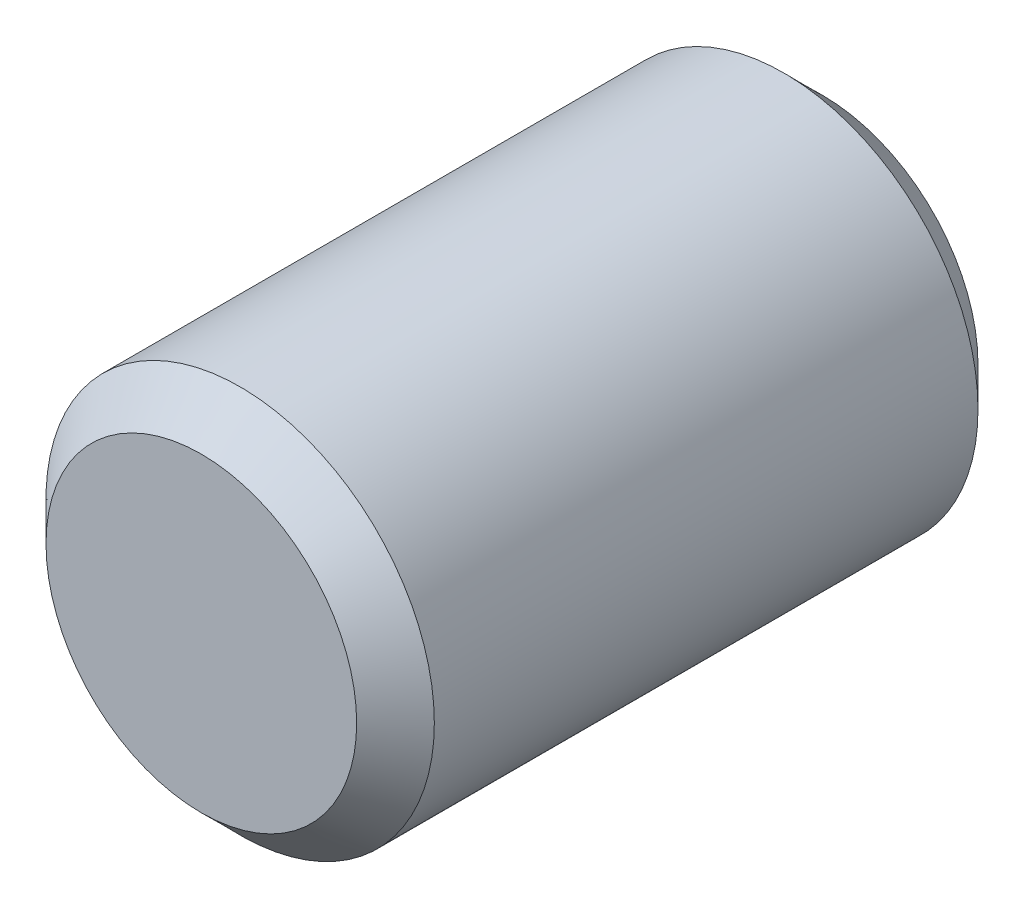
from build123d import *

# Parameters (mm, degrees)
PIN_PROFILE_5_R          = 2.5
PIN_BODY_5X8_DEPTH       = 8
END_CHAMFERS_0_5X45_SIZE = 0.5


with BuildPart() as part:
    # Pin Profile Ø5 → Pin Body Ø5x8 (new body)
    with BuildSketch(Plane.XY):
        Circle(PIN_PROFILE_5_R)
    extrude(amount=PIN_BODY_5X8_DEPTH)

    # End Chamfers 0.5x45°
    end_chamfers_0_5x45_edges = [part.edges().sort_by_distance(p)[0] for p in [
        (-2.5, 0, 0),
        (-2.5, 0, 8),
    ]]
    chamfer(end_chamfers_0_5x45_edges, length=END_CHAMFERS_0_5X45_SIZE)


solid = part.part
